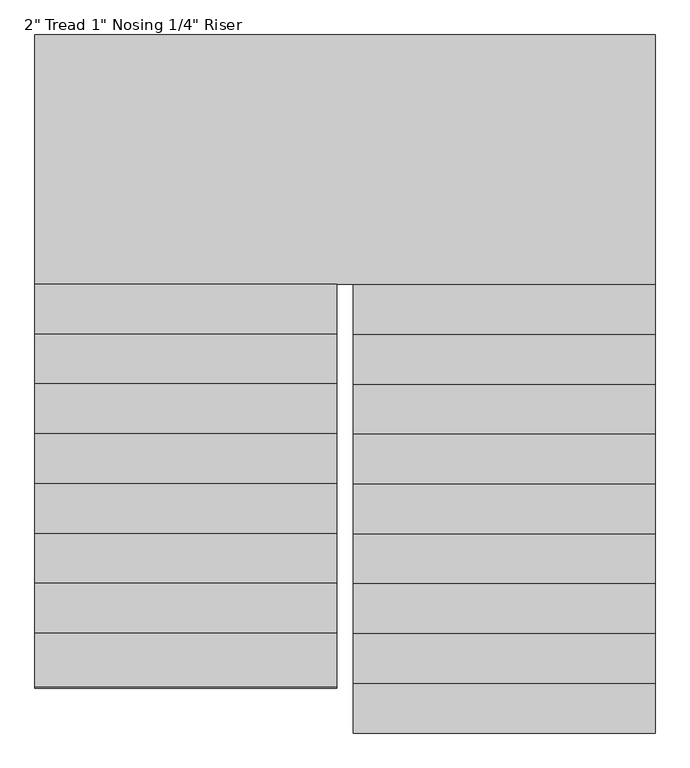
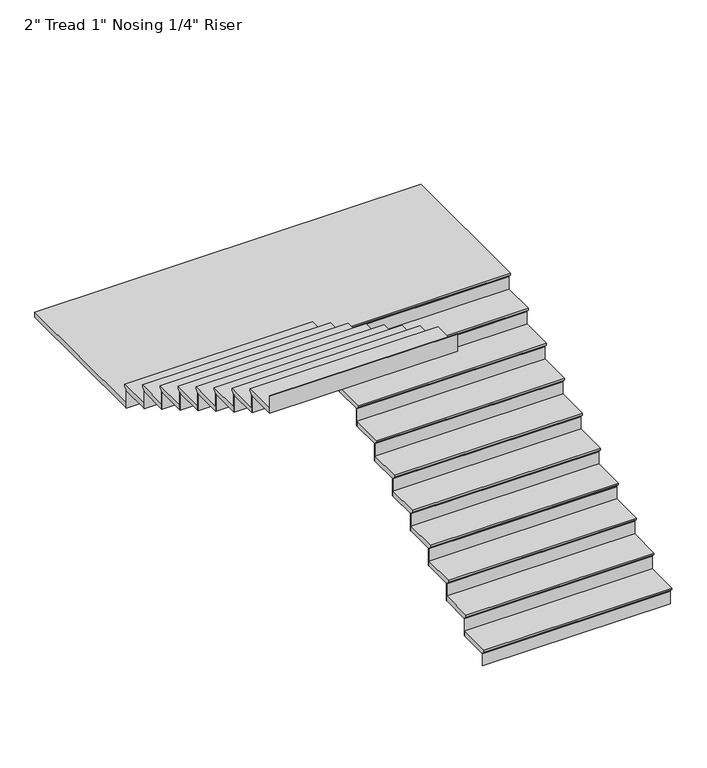
"""IFC4 building model written with IfcOpenShell, lengths in millimetres: stair flight geometry."""

from ifc_helpers import new_model, si_unit, origin, place, context, project, spatial, faceted_brep, source, transform, mapped, element, save


def stair_flight_26a2e14d(model_context):
    return source(origin(), model_context, "Body", "Brep", [
        faceted_brep([(7785.2813124, -8648.1976656, 920.75), (7785.2813124, -8648.1976656, 939.8), (5940.6255016, -8648.1976656, 939.8), (5940.6255016, -8648.1976656, 920.75), (7785.2813124, -8622.7976656, 895.35), (5940.6255016, -8622.7976656, 895.35), (7785.2813124, -8317.9976656, 939.8), (5940.6255016, -8317.9976656, 939.8), (5940.6255016, -8622.7976656, 889.0), (5940.6255016, -8317.9976656, 889.0), (7785.2813124, -8317.9976656, 889.0), (7785.2813124, -8622.7976656, 889.0)], [[[0, 1, 2, 3]], [[4, 0, 3, 5]], [[2, 1, 6, 7]], [[8, 9, 10, 11]], [[2, 7, 9, 8, 5, 3]], [[8, 11, 4, 5]], [[6, 1, 0, 4, 11, 10]], [[7, 6, 10, 9]]]),
        faceted_brep([(7785.2813124, -8622.7976656, 889.0), (7785.2813124, -8622.7976656, 762.0), (7785.2813124, -8616.4476656, 762.0), (7785.2813124, -8616.4476656, 889.0), (5940.6255016, -8622.7976656, 889.0), (5940.6255016, -8616.4476656, 889.0), (5940.6255016, -8616.4476656, 762.0), (5940.6255016, -8622.7976656, 762.0)], [[[0, 1, 2, 3]], [[4, 5, 6, 7]], [[1, 0, 4, 7]], [[2, 1, 7, 6]], [[3, 2, 6, 5]], [[0, 3, 5, 4]]]),
        faceted_brep([(7785.2813124, -8317.9976656, 1066.8), (7785.2813124, -8317.9976656, 889.0), (7785.2813124, -8311.6476656, 889.0), (7785.2813124, -8311.6476656, 1066.8), (5940.6255016, -8317.9976656, 1066.8), (5940.6255016, -8311.6476656, 1066.8), (5940.6255016, -8311.6476656, 889.0), (5940.6255016, -8317.9976656, 889.0)], [[[0, 1, 2, 3]], [[4, 5, 6, 7]], [[1, 0, 4, 7]], [[2, 1, 7, 6]], [[3, 2, 6, 5]], [[0, 3, 5, 4]]]),
        faceted_brep([(5940.6255016, -8343.3976656, 1117.6), (7785.2813124, -8343.3976656, 1117.6), (7785.2813124, -8013.1976656, 1117.6), (5940.6255016, -8013.1976656, 1117.6), (5940.6255016, -8317.9976656, 1066.8), (5940.6255016, -8013.1976656, 1066.8), (7785.2813124, -8013.1976656, 1066.8), (7785.2813124, -8317.9976656, 1066.8), (5940.6255016, -8317.9976656, 1073.15), (5940.6255016, -8343.3976656, 1098.55), (7785.2813124, -8317.9976656, 1073.15), (7785.2813124, -8343.3976656, 1098.55)], [[[0, 1, 2, 3]], [[4, 5, 6, 7]], [[0, 3, 5, 4, 8, 9]], [[4, 7, 10, 8]], [[2, 1, 11, 10, 7, 6]], [[3, 2, 6, 5]], [[11, 1, 0, 9]], [[10, 11, 9, 8]]]),
        faceted_brep([(7785.2813124, -8013.1976656, 1244.6), (7785.2813124, -8013.1976656, 1066.8), (7785.2813124, -8006.8476656, 1066.8), (7785.2813124, -8006.8476656, 1244.6), (5940.6255016, -8013.1976656, 1244.6), (5940.6255016, -8006.8476656, 1244.6), (5940.6255016, -8006.8476656, 1066.8), (5940.6255016, -8013.1976656, 1066.8)], [[[0, 1, 2, 3]], [[4, 5, 6, 7]], [[1, 0, 4, 7]], [[2, 1, 7, 6]], [[3, 2, 6, 5]], [[0, 3, 5, 4]]]),
        faceted_brep([(5940.6255016, -8038.5976656, 1295.4), (7785.2813124, -8038.5976656, 1295.4), (7785.2813124, -7708.3976656, 1295.4), (5940.6255016, -7708.3976656, 1295.4), (5940.6255016, -8013.1976656, 1244.6), (5940.6255016, -7708.3976656, 1244.6), (7785.2813124, -7708.3976656, 1244.6), (7785.2813124, -8013.1976656, 1244.6), (5940.6255016, -8013.1976656, 1250.95), (5940.6255016, -8038.5976656, 1276.35), (7785.2813124, -8013.1976656, 1250.95), (7785.2813124, -8038.5976656, 1276.35)], [[[0, 1, 2, 3]], [[4, 5, 6, 7]], [[0, 3, 5, 4, 8, 9]], [[4, 7, 10, 8]], [[2, 1, 11, 10, 7, 6]], [[3, 2, 6, 5]], [[11, 1, 0, 9]], [[10, 11, 9, 8]]]),
        faceted_brep([(7785.2813124, -7708.3976656, 1422.4), (7785.2813124, -7708.3976656, 1244.6), (7785.2813124, -7702.0476656, 1244.6), (7785.2813124, -7702.0476656, 1422.4), (5940.6255016, -7708.3976656, 1422.4), (5940.6255016, -7702.0476656, 1422.4), (5940.6255016, -7702.0476656, 1244.6), (5940.6255016, -7708.3976656, 1244.6)], [[[0, 1, 2, 3]], [[4, 5, 6, 7]], [[1, 0, 4, 7]], [[2, 1, 7, 6]], [[3, 2, 6, 5]], [[0, 3, 5, 4]]]),
        faceted_brep([(5940.6255016, -7733.7976656, 1473.2), (7785.2813124, -7733.7976656, 1473.2), (7785.2813124, -7403.5976656, 1473.2), (5940.6255016, -7403.5976656, 1473.2), (5940.6255016, -7708.3976656, 1422.4), (5940.6255016, -7403.5976656, 1422.4), (7785.2813124, -7403.5976656, 1422.4), (7785.2813124, -7708.3976656, 1422.4), (5940.6255016, -7708.3976656, 1428.75), (5940.6255016, -7733.7976656, 1454.15), (7785.2813124, -7708.3976656, 1428.75), (7785.2813124, -7733.7976656, 1454.15)], [[[0, 1, 2, 3]], [[4, 5, 6, 7]], [[0, 3, 5, 4, 8, 9]], [[4, 7, 10, 8]], [[2, 1, 11, 10, 7, 6]], [[3, 2, 6, 5]], [[11, 1, 0, 9]], [[10, 11, 9, 8]]]),
        faceted_brep([(7785.2813124, -7403.5976656, 1600.2), (7785.2813124, -7403.5976656, 1422.4), (7785.2813124, -7397.2476656, 1422.4), (7785.2813124, -7397.2476656, 1600.2), (5940.6255016, -7403.5976656, 1600.2), (5940.6255016, -7397.2476656, 1600.2), (5940.6255016, -7397.2476656, 1422.4), (5940.6255016, -7403.5976656, 1422.4)], [[[0, 1, 2, 3]], [[4, 5, 6, 7]], [[1, 0, 4, 7]], [[2, 1, 7, 6]], [[3, 2, 6, 5]], [[0, 3, 5, 4]]]),
        faceted_brep([(5940.6255016, -7428.9976656, 1651.0), (7785.2813124, -7428.9976656, 1651.0), (7785.2813124, -7098.7976656, 1651.0), (5940.6255016, -7098.7976656, 1651.0), (5940.6255016, -7403.5976656, 1600.2), (5940.6255016, -7098.7976656, 1600.2), (7785.2813124, -7098.7976656, 1600.2), (7785.2813124, -7403.5976656, 1600.2), (5940.6255016, -7403.5976656, 1606.55), (5940.6255016, -7428.9976656, 1631.95), (7785.2813124, -7403.5976656, 1606.55), (7785.2813124, -7428.9976656, 1631.95)], [[[0, 1, 2, 3]], [[4, 5, 6, 7]], [[0, 3, 5, 4, 8, 9]], [[4, 7, 10, 8]], [[2, 1, 11, 10, 7, 6]], [[3, 2, 6, 5]], [[11, 1, 0, 9]], [[10, 11, 9, 8]]]),
        faceted_brep([(7785.2813124, -7098.7976656, 1778.0), (7785.2813124, -7098.7976656, 1600.2), (7785.2813124, -7092.4476656, 1600.2), (7785.2813124, -7092.4476656, 1778.0), (5940.6255016, -7098.7976656, 1778.0), (5940.6255016, -7092.4476656, 1778.0), (5940.6255016, -7092.4476656, 1600.2), (5940.6255016, -7098.7976656, 1600.2)], [[[0, 1, 2, 3]], [[4, 5, 6, 7]], [[1, 0, 4, 7]], [[2, 1, 7, 6]], [[3, 2, 6, 5]], [[0, 3, 5, 4]]]),
        faceted_brep([(5940.6255016, -7124.1976656, 1828.8), (7785.2813124, -7124.1976656, 1828.8), (7785.2813124, -6793.9976656, 1828.8), (5940.6255016, -6793.9976656, 1828.8), (5940.6255016, -7098.7976656, 1778.0), (5940.6255016, -6793.9976656, 1778.0), (7785.2813124, -6793.9976656, 1778.0), (7785.2813124, -7098.7976656, 1778.0), (5940.6255016, -7098.7976656, 1784.35), (5940.6255016, -7124.1976656, 1809.75), (7785.2813124, -7098.7976656, 1784.35), (7785.2813124, -7124.1976656, 1809.75)], [[[0, 1, 2, 3]], [[4, 5, 6, 7]], [[0, 3, 5, 4, 8, 9]], [[4, 7, 10, 8]], [[2, 1, 11, 10, 7, 6]], [[3, 2, 6, 5]], [[11, 1, 0, 9]], [[10, 11, 9, 8]]]),
        faceted_brep([(7785.2813124, -6793.9976656, 1955.8), (7785.2813124, -6793.9976656, 1778.0), (7785.2813124, -6787.6476656, 1778.0), (7785.2813124, -6787.6476656, 1955.8), (5940.6255016, -6793.9976656, 1955.8), (5940.6255016, -6787.6476656, 1955.8), (5940.6255016, -6787.6476656, 1778.0), (5940.6255016, -6793.9976656, 1778.0)], [[[0, 1, 2, 3]], [[4, 5, 6, 7]], [[1, 0, 4, 7]], [[2, 1, 7, 6]], [[3, 2, 6, 5]], [[0, 3, 5, 4]]]),
        faceted_brep([(5940.6255016, -6819.3976656, 2006.6), (7785.2813124, -6819.3976656, 2006.6), (7785.2813124, -6489.1976656, 2006.6), (5940.6255016, -6489.1976656, 2006.6), (5940.6255016, -6793.9976656, 1955.8), (5940.6255016, -6489.1976656, 1955.8), (7785.2813124, -6489.1976656, 1955.8), (7785.2813124, -6793.9976656, 1955.8), (5940.6255016, -6793.9976656, 1962.15), (5940.6255016, -6819.3976656, 1987.55), (7785.2813124, -6793.9976656, 1962.15), (7785.2813124, -6819.3976656, 1987.55)], [[[0, 1, 2, 3]], [[4, 5, 6, 7]], [[0, 3, 5, 4, 8, 9]], [[4, 7, 10, 8]], [[2, 1, 11, 10, 7, 6]], [[3, 2, 6, 5]], [[11, 1, 0, 9]], [[10, 11, 9, 8]]]),
        faceted_brep([(7785.2813124, -6489.1976656, 2133.6), (7785.2813124, -6489.1976656, 1955.8), (7785.2813124, -6482.8476656, 1955.8), (7785.2813124, -6482.8476656, 2133.6), (5940.6255016, -6489.1976656, 2133.6), (5940.6255016, -6482.8476656, 2133.6), (5940.6255016, -6482.8476656, 1955.8), (5940.6255016, -6489.1976656, 1955.8)], [[[0, 1, 2, 3]], [[4, 5, 6, 7]], [[1, 0, 4, 7]], [[2, 1, 7, 6]], [[3, 2, 6, 5]], [[0, 3, 5, 4]]]),
        faceted_brep([(5940.6255016, -6514.5976656, 2184.4), (7785.2813124, -6514.5976656, 2184.4), (7785.2813124, -6184.3976656, 2184.4), (5940.6255016, -6184.3976656, 2184.4), (5940.6255016, -6489.1976656, 2133.6), (5940.6255016, -6184.3976656, 2133.6), (7785.2813124, -6184.3976656, 2133.6), (7785.2813124, -6489.1976656, 2133.6), (5940.6255016, -6489.1976656, 2139.95), (5940.6255016, -6514.5976656, 2165.35), (7785.2813124, -6489.1976656, 2139.95), (7785.2813124, -6514.5976656, 2165.35)], [[[0, 1, 2, 3]], [[4, 5, 6, 7]], [[0, 3, 5, 4, 8, 9]], [[4, 7, 10, 8]], [[2, 1, 11, 10, 7, 6]], [[3, 2, 6, 5]], [[11, 1, 0, 9]], [[10, 11, 9, 8]]]),
        faceted_brep([(7785.2813124, -5879.5976656, 2489.2), (7785.2813124, -5879.5976656, 2311.4), (7785.2813124, -5873.2476656, 2311.4), (7785.2813124, -5873.2476656, 2489.2), (5940.6255016, -5879.5976656, 2489.2), (5940.6255016, -5873.2476656, 2489.2), (5940.6255016, -5873.2476656, 2311.4), (5940.6255016, -5879.5976656, 2311.4)], [[[0, 1, 2, 3]], [[4, 5, 6, 7]], [[1, 0, 4, 7]], [[2, 1, 7, 6]], [[3, 2, 6, 5]], [[0, 3, 5, 4]]]),
        faceted_brep([(5839.0255016, -5930.3976656, 2540.0), (5839.0255016, -5904.9976656, 2540.0), (7785.2813124, -5904.9976656, 2540.0), (7785.2813124, -4380.9976656, 2540.0), (3994.3696908, -4380.9976656, 2540.0), (3994.3696908, -5930.3976656, 2540.0), (5839.0255016, -5904.9976656, 2489.2), (5839.0255016, -5930.3976656, 2489.2), (3994.3696908, -5930.3976656, 2489.2), (3994.3696908, -4380.9976656, 2489.2), (7785.2813124, -4380.9976656, 2489.2), (7785.2813124, -5879.5976656, 2489.2), (5940.6255016, -5879.5976656, 2489.2), (5940.6255016, -5904.9976656, 2489.2), (7785.2813124, -5879.5976656, 2495.55), (5940.6255016, -5879.5976656, 2495.55), (7785.2813124, -5904.9976656, 2520.95), (5940.6255016, -5904.9976656, 2520.95)], [[[0, 1, 2, 3, 4, 5]], [[6, 7, 8, 9, 10, 11, 12, 13]], [[1, 0, 7, 6]], [[12, 11, 14, 15]], [[3, 2, 16, 14, 11, 10]], [[0, 5, 8, 7]], [[14, 16, 17, 15]], [[2, 1, 6, 13, 17, 16]], [[13, 12, 15, 17]], [[4, 3, 10, 9]], [[5, 4, 9, 8]]]),
        faceted_brep([(3994.3696908, -8368.7976656, 4089.4), (3994.3696908, -8368.7976656, 3911.6), (3994.3696908, -8375.1476656, 3911.6), (3994.3696908, -8375.1476656, 4089.4), (5839.0255016, -8368.7976656, 4089.4), (5839.0255016, -8375.1476656, 4089.4), (5839.0255016, -8375.1476656, 3911.6), (5839.0255016, -8368.7976656, 3911.6)], [[[0, 1, 2, 3]], [[4, 5, 6, 7]], [[1, 0, 4, 7]], [[2, 1, 7, 6]], [[3, 2, 6, 5]], [[0, 3, 5, 4]]]),
        faceted_brep([(7785.2813124, -6184.3976656, 2311.4), (7785.2813124, -6184.3976656, 2133.6), (7785.2813124, -6178.0476656, 2133.6), (7785.2813124, -6178.0476656, 2311.4), (5940.6255016, -6184.3976656, 2311.4), (5940.6255016, -6178.0476656, 2311.4), (5940.6255016, -6178.0476656, 2133.6), (5940.6255016, -6184.3976656, 2133.6)], [[[0, 1, 2, 3]], [[4, 5, 6, 7]], [[1, 0, 4, 7]], [[2, 1, 7, 6]], [[3, 2, 6, 5]], [[0, 3, 5, 4]]]),
        faceted_brep([(5940.6255016, -6209.7976656, 2362.2), (7785.2813124, -6209.7976656, 2362.2), (7785.2813124, -5879.5976656, 2362.2), (5940.6255016, -5879.5976656, 2362.2), (5940.6255016, -6184.3976656, 2311.4), (5940.6255016, -5879.5976656, 2311.4), (7785.2813124, -5879.5976656, 2311.4), (7785.2813124, -6184.3976656, 2311.4), (5940.6255016, -6184.3976656, 2317.75), (5940.6255016, -6209.7976656, 2343.15), (7785.2813124, -6184.3976656, 2317.75), (7785.2813124, -6209.7976656, 2343.15)], [[[0, 1, 2, 3]], [[4, 5, 6, 7]], [[0, 3, 5, 4, 8, 9]], [[4, 7, 10, 8]], [[2, 1, 11, 10, 7, 6]], [[3, 2, 6, 5]], [[11, 1, 0, 9]], [[10, 11, 9, 8]]]),
        faceted_brep([(3994.3696908, -5930.3976656, 2667.0), (3994.3696908, -5930.3976656, 2489.2), (3994.3696908, -5936.7476656, 2489.2), (3994.3696908, -5936.7476656, 2667.0), (5839.0255016, -5930.3976656, 2667.0), (5839.0255016, -5936.7476656, 2667.0), (5839.0255016, -5936.7476656, 2489.2), (5839.0255016, -5930.3976656, 2489.2)], [[[0, 1, 2, 3]], [[4, 5, 6, 7]], [[1, 0, 4, 7]], [[2, 1, 7, 6]], [[3, 2, 6, 5]], [[0, 3, 5, 4]]]),
        faceted_brep([(5839.0255016, -5904.9976656, 2717.8), (3994.3696908, -5904.9976656, 2717.8), (3994.3696908, -6235.1976656, 2717.8), (5839.0255016, -6235.1976656, 2717.8), (5839.0255016, -5930.3976656, 2667.0), (5839.0255016, -6235.1976656, 2667.0), (3994.3696908, -6235.1976656, 2667.0), (3994.3696908, -5930.3976656, 2667.0), (5839.0255016, -5930.3976656, 2673.35), (5839.0255016, -5904.9976656, 2698.75), (3994.3696908, -5930.3976656, 2673.35), (3994.3696908, -5904.9976656, 2698.75)], [[[0, 1, 2, 3]], [[4, 5, 6, 7]], [[0, 3, 5, 4, 8, 9]], [[4, 7, 10, 8]], [[2, 1, 11, 10, 7, 6]], [[3, 2, 6, 5]], [[11, 1, 0, 9]], [[10, 11, 9, 8]]]),
        faceted_brep([(3994.3696908, -6235.1976656, 2844.8), (3994.3696908, -6235.1976656, 2667.0), (3994.3696908, -6241.5476656, 2667.0), (3994.3696908, -6241.5476656, 2844.8), (5839.0255016, -6235.1976656, 2844.8), (5839.0255016, -6241.5476656, 2844.8), (5839.0255016, -6241.5476656, 2667.0), (5839.0255016, -6235.1976656, 2667.0)], [[[0, 1, 2, 3]], [[4, 5, 6, 7]], [[1, 0, 4, 7]], [[2, 1, 7, 6]], [[3, 2, 6, 5]], [[0, 3, 5, 4]]]),
        faceted_brep([(5839.0255016, -6209.7976656, 2895.6), (3994.3696908, -6209.7976656, 2895.6), (3994.3696908, -6539.9976656, 2895.6), (5839.0255016, -6539.9976656, 2895.6), (5839.0255016, -6235.1976656, 2844.8), (5839.0255016, -6539.9976656, 2844.8), (3994.3696908, -6539.9976656, 2844.8), (3994.3696908, -6235.1976656, 2844.8), (5839.0255016, -6235.1976656, 2851.15), (5839.0255016, -6209.7976656, 2876.55), (3994.3696908, -6235.1976656, 2851.15), (3994.3696908, -6209.7976656, 2876.55)], [[[0, 1, 2, 3]], [[4, 5, 6, 7]], [[0, 3, 5, 4, 8, 9]], [[4, 7, 10, 8]], [[2, 1, 11, 10, 7, 6]], [[3, 2, 6, 5]], [[11, 1, 0, 9]], [[10, 11, 9, 8]]]),
        faceted_brep([(3994.3696908, -6539.9976656, 3022.6), (3994.3696908, -6539.9976656, 2844.8), (3994.3696908, -6546.3476656, 2844.8), (3994.3696908, -6546.3476656, 3022.6), (5839.0255016, -6539.9976656, 3022.6), (5839.0255016, -6546.3476656, 3022.6), (5839.0255016, -6546.3476656, 2844.8), (5839.0255016, -6539.9976656, 2844.8)], [[[0, 1, 2, 3]], [[4, 5, 6, 7]], [[1, 0, 4, 7]], [[2, 1, 7, 6]], [[3, 2, 6, 5]], [[0, 3, 5, 4]]]),
        faceted_brep([(5839.0255016, -6514.5976656, 3073.4), (3994.3696908, -6514.5976656, 3073.4), (3994.3696908, -6844.7976656, 3073.4), (5839.0255016, -6844.7976656, 3073.4), (5839.0255016, -6539.9976656, 3022.6), (5839.0255016, -6844.7976656, 3022.6), (3994.3696908, -6844.7976656, 3022.6), (3994.3696908, -6539.9976656, 3022.6), (5839.0255016, -6539.9976656, 3028.95), (5839.0255016, -6514.5976656, 3054.35), (3994.3696908, -6539.9976656, 3028.95), (3994.3696908, -6514.5976656, 3054.35)], [[[0, 1, 2, 3]], [[4, 5, 6, 7]], [[0, 3, 5, 4, 8, 9]], [[4, 7, 10, 8]], [[2, 1, 11, 10, 7, 6]], [[3, 2, 6, 5]], [[11, 1, 0, 9]], [[10, 11, 9, 8]]]),
        faceted_brep([(3994.3696908, -6844.7976656, 3200.4), (3994.3696908, -6844.7976656, 3022.6), (3994.3696908, -6851.1476656, 3022.6), (3994.3696908, -6851.1476656, 3200.4), (5839.0255016, -6844.7976656, 3200.4), (5839.0255016, -6851.1476656, 3200.4), (5839.0255016, -6851.1476656, 3022.6), (5839.0255016, -6844.7976656, 3022.6)], [[[0, 1, 2, 3]], [[4, 5, 6, 7]], [[1, 0, 4, 7]], [[2, 1, 7, 6]], [[3, 2, 6, 5]], [[0, 3, 5, 4]]]),
        faceted_brep([(5839.0255016, -6819.3976656, 3251.2), (3994.3696908, -6819.3976656, 3251.2), (3994.3696908, -7149.5976656, 3251.2), (5839.0255016, -7149.5976656, 3251.2), (5839.0255016, -6844.7976656, 3200.4), (5839.0255016, -7149.5976656, 3200.4), (3994.3696908, -7149.5976656, 3200.4), (3994.3696908, -6844.7976656, 3200.4), (5839.0255016, -6844.7976656, 3206.75), (5839.0255016, -6819.3976656, 3232.15), (3994.3696908, -6844.7976656, 3206.75), (3994.3696908, -6819.3976656, 3232.15)], [[[0, 1, 2, 3]], [[4, 5, 6, 7]], [[0, 3, 5, 4, 8, 9]], [[4, 7, 10, 8]], [[2, 1, 11, 10, 7, 6]], [[3, 2, 6, 5]], [[11, 1, 0, 9]], [[10, 11, 9, 8]]]),
        faceted_brep([(3994.3696908, -7149.5976656, 3378.2), (3994.3696908, -7149.5976656, 3200.4), (3994.3696908, -7155.9476656, 3200.4), (3994.3696908, -7155.9476656, 3378.2), (5839.0255016, -7149.5976656, 3378.2), (5839.0255016, -7155.9476656, 3378.2), (5839.0255016, -7155.9476656, 3200.4), (5839.0255016, -7149.5976656, 3200.4)], [[[0, 1, 2, 3]], [[4, 5, 6, 7]], [[1, 0, 4, 7]], [[2, 1, 7, 6]], [[3, 2, 6, 5]], [[0, 3, 5, 4]]]),
        faceted_brep([(5839.0255016, -7124.1976656, 3429.0), (3994.3696908, -7124.1976656, 3429.0), (3994.3696908, -7454.3976656, 3429.0), (5839.0255016, -7454.3976656, 3429.0), (5839.0255016, -7149.5976656, 3378.2), (5839.0255016, -7454.3976656, 3378.2), (3994.3696908, -7454.3976656, 3378.2), (3994.3696908, -7149.5976656, 3378.2), (5839.0255016, -7149.5976656, 3384.55), (5839.0255016, -7124.1976656, 3409.95), (3994.3696908, -7149.5976656, 3384.55), (3994.3696908, -7124.1976656, 3409.95)], [[[0, 1, 2, 3]], [[4, 5, 6, 7]], [[0, 3, 5, 4, 8, 9]], [[4, 7, 10, 8]], [[2, 1, 11, 10, 7, 6]], [[3, 2, 6, 5]], [[11, 1, 0, 9]], [[10, 11, 9, 8]]]),
        faceted_brep([(3994.3696908, -7454.3976656, 3556.0), (3994.3696908, -7454.3976656, 3378.2), (3994.3696908, -7460.7476656, 3378.2), (3994.3696908, -7460.7476656, 3556.0), (5839.0255016, -7454.3976656, 3556.0), (5839.0255016, -7460.7476656, 3556.0), (5839.0255016, -7460.7476656, 3378.2), (5839.0255016, -7454.3976656, 3378.2)], [[[0, 1, 2, 3]], [[4, 5, 6, 7]], [[1, 0, 4, 7]], [[2, 1, 7, 6]], [[3, 2, 6, 5]], [[0, 3, 5, 4]]]),
        faceted_brep([(5839.0255016, -7428.9976656, 3606.8), (3994.3696908, -7428.9976656, 3606.8), (3994.3696908, -7759.1976656, 3606.8), (5839.0255016, -7759.1976656, 3606.8), (5839.0255016, -7454.3976656, 3556.0), (5839.0255016, -7759.1976656, 3556.0), (3994.3696908, -7759.1976656, 3556.0), (3994.3696908, -7454.3976656, 3556.0), (5839.0255016, -7454.3976656, 3562.35), (5839.0255016, -7428.9976656, 3587.75), (3994.3696908, -7454.3976656, 3562.35), (3994.3696908, -7428.9976656, 3587.75)], [[[0, 1, 2, 3]], [[4, 5, 6, 7]], [[0, 3, 5, 4, 8, 9]], [[4, 7, 10, 8]], [[2, 1, 11, 10, 7, 6]], [[3, 2, 6, 5]], [[11, 1, 0, 9]], [[10, 11, 9, 8]]]),
        faceted_brep([(3994.3696908, -7759.1976656, 3733.8), (3994.3696908, -7759.1976656, 3556.0), (3994.3696908, -7765.5476656, 3556.0), (3994.3696908, -7765.5476656, 3733.8), (5839.0255016, -7759.1976656, 3733.8), (5839.0255016, -7765.5476656, 3733.8), (5839.0255016, -7765.5476656, 3556.0), (5839.0255016, -7759.1976656, 3556.0)], [[[0, 1, 2, 3]], [[4, 5, 6, 7]], [[1, 0, 4, 7]], [[2, 1, 7, 6]], [[3, 2, 6, 5]], [[0, 3, 5, 4]]]),
        faceted_brep([(5839.0255016, -7733.7976656, 3784.6), (3994.3696908, -7733.7976656, 3784.6), (3994.3696908, -8063.9976656, 3784.6), (5839.0255016, -8063.9976656, 3784.6), (5839.0255016, -7759.1976656, 3733.8), (5839.0255016, -8063.9976656, 3733.8), (3994.3696908, -8063.9976656, 3733.8), (3994.3696908, -7759.1976656, 3733.8), (5839.0255016, -7759.1976656, 3740.15), (5839.0255016, -7733.7976656, 3765.55), (3994.3696908, -7759.1976656, 3740.15), (3994.3696908, -7733.7976656, 3765.55)], [[[0, 1, 2, 3]], [[4, 5, 6, 7]], [[0, 3, 5, 4, 8, 9]], [[4, 7, 10, 8]], [[2, 1, 11, 10, 7, 6]], [[3, 2, 6, 5]], [[11, 1, 0, 9]], [[10, 11, 9, 8]]]),
        faceted_brep([(3994.3696908, -8063.9976656, 3911.6), (3994.3696908, -8063.9976656, 3733.8), (3994.3696908, -8070.3476656, 3733.8), (3994.3696908, -8070.3476656, 3911.6), (5839.0255016, -8063.9976656, 3911.6), (5839.0255016, -8070.3476656, 3911.6), (5839.0255016, -8070.3476656, 3733.8), (5839.0255016, -8063.9976656, 3733.8)], [[[0, 1, 2, 3]], [[4, 5, 6, 7]], [[1, 0, 4, 7]], [[2, 1, 7, 6]], [[3, 2, 6, 5]], [[0, 3, 5, 4]]]),
        faceted_brep([(5839.0255016, -8038.5976656, 3962.4), (3994.3696908, -8038.5976656, 3962.4), (3994.3696908, -8368.7976656, 3962.4), (5839.0255016, -8368.7976656, 3962.4), (5839.0255016, -8063.9976656, 3911.6), (5839.0255016, -8368.7976656, 3911.6), (3994.3696908, -8368.7976656, 3911.6), (3994.3696908, -8063.9976656, 3911.6), (5839.0255016, -8063.9976656, 3917.95), (5839.0255016, -8038.5976656, 3943.35), (3994.3696908, -8063.9976656, 3917.95), (3994.3696908, -8038.5976656, 3943.35)], [[[0, 1, 2, 3]], [[4, 5, 6, 7]], [[0, 3, 5, 4, 8, 9]], [[4, 7, 10, 8]], [[2, 1, 11, 10, 7, 6]], [[3, 2, 6, 5]], [[11, 1, 0, 9]], [[10, 11, 9, 8]]]),
    ])


if __name__ == "__main__":
    model = new_model("IFC4")
    model_context = context("Model", 3, world=origin())
    ifc_project = project(units=[si_unit("LENGTHUNIT", "METRE", prefix="MILLI")], contexts=[model_context])
    site = spatial("IfcSite", under=ifc_project)
    building = spatial("IfcBuilding", under=site)
    placement = place(None, origin())
    stair_flight_shape = stair_flight_26a2e14d(model_context)
    element("IfcStairFlight", 1, ObjectType="2\" Tread 1\" Nosing 1/4\" Riser", at=placement, inside=building, context=model_context, shape_type="MappedRepresentation", body=[
        mapped(stair_flight_shape, transform((0.0, 0.0, 0.0), x_axis=(1.0, 0.0, 0.0), y_axis=(0.0, 1.0, 0.0), z_axis=(0.0, 0.0, 1.0))),
    ])
    save(model, "model.ifc")
